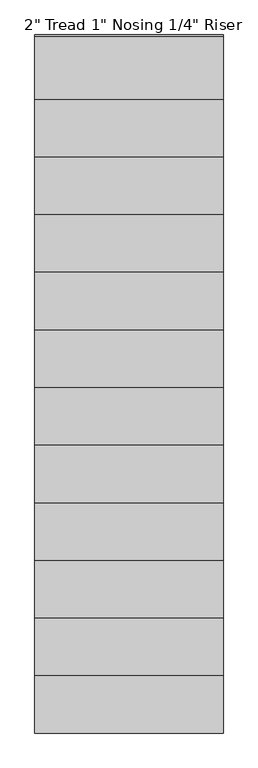
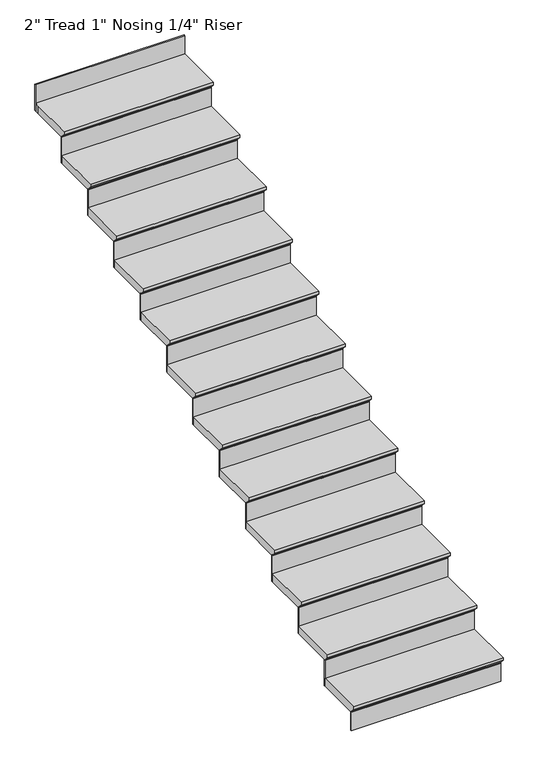
"""IFC4 building model written with IfcOpenShell, lengths in millimetres: stair flight geometry."""

from ifc_helpers import new_model, si_unit, origin, place, context, project, spatial, faceted_brep, source, transform, mapped, element, save


def stair_flight_fc83273d(model_context):
    return source(origin(), model_context, "Body", "Brep", [
        faceted_brep([(-2703.0415084, 19841.9216096, 49768.9005799), (-2703.0415084, 19841.9216096, 49787.9505799), (-3617.4415084, 19841.9216096, 49787.9505799), (-3617.4415084, 19841.9216096, 49768.9005799), (-2703.0415084, 19867.3216096, 49743.5005799), (-3617.4415084, 19867.3216096, 49743.5005799), (-2703.0415084, 20146.7216096, 49787.9505799), (-3617.4415084, 20146.7216096, 49787.9505799), (-3617.4415084, 19867.3216096, 49737.1505799), (-3617.4415084, 20146.7216096, 49737.1505799), (-2703.0415084, 20146.7216096, 49737.1505799), (-2703.0415084, 19867.3216096, 49737.1505799)], [[[0, 1, 2, 3]], [[4, 0, 3, 5]], [[2, 1, 6, 7]], [[8, 9, 10, 11]], [[2, 7, 9, 8, 5, 3]], [[8, 11, 4, 5]], [[6, 1, 0, 4, 11, 10]], [[7, 6, 10, 9]]]),
        faceted_brep([(-2703.0415084, 19867.3216096, 49737.1505799), (-2703.0415084, 19867.3216096, 49618.6172466), (-2703.0415084, 19873.6716096, 49618.6172466), (-2703.0415084, 19873.6716096, 49737.1505799), (-3617.4415084, 19867.3216096, 49737.1505799), (-3617.4415084, 19873.6716096, 49737.1505799), (-3617.4415084, 19873.6716096, 49618.6172466), (-3617.4415084, 19867.3216096, 49618.6172466)], [[[0, 1, 2, 3]], [[4, 5, 6, 7]], [[1, 0, 4, 7]], [[2, 1, 7, 6]], [[3, 2, 6, 5]], [[0, 3, 5, 4]]]),
        faceted_brep([(-2703.0415084, 20146.7216096, 49906.4839133), (-2703.0415084, 20146.7216096, 49737.1505799), (-2703.0415084, 20153.0716096, 49737.1505799), (-2703.0415084, 20153.0716096, 49906.4839133), (-3617.4415084, 20146.7216096, 49906.4839133), (-3617.4415084, 20153.0716096, 49906.4839133), (-3617.4415084, 20153.0716096, 49737.1505799), (-3617.4415084, 20146.7216096, 49737.1505799)], [[[0, 1, 2, 3]], [[4, 5, 6, 7]], [[1, 0, 4, 7]], [[2, 1, 7, 6]], [[3, 2, 6, 5]], [[0, 3, 5, 4]]]),
        faceted_brep([(-3617.4415084, 20121.3216096, 49957.2839133), (-2703.0415084, 20121.3216096, 49957.2839133), (-2703.0415084, 20426.1216096, 49957.2839133), (-3617.4415084, 20426.1216096, 49957.2839133), (-3617.4415084, 20146.7216096, 49906.4839133), (-3617.4415084, 20426.1216096, 49906.4839133), (-2703.0415084, 20426.1216096, 49906.4839133), (-2703.0415084, 20146.7216096, 49906.4839133), (-3617.4415084, 20146.7216096, 49912.8339133), (-3617.4415084, 20121.3216096, 49938.2339133), (-2703.0415084, 20146.7216096, 49912.8339133), (-2703.0415084, 20121.3216096, 49938.2339133)], [[[0, 1, 2, 3]], [[4, 5, 6, 7]], [[0, 3, 5, 4, 8, 9]], [[4, 7, 10, 8]], [[2, 1, 11, 10, 7, 6]], [[3, 2, 6, 5]], [[11, 1, 0, 9]], [[10, 11, 9, 8]]]),
        faceted_brep([(-2703.0415084, 20426.1216096, 50075.8172466), (-2703.0415084, 20426.1216096, 49906.4839133), (-2703.0415084, 20432.4716096, 49906.4839133), (-2703.0415084, 20432.4716096, 50075.8172466), (-3617.4415084, 20426.1216096, 50075.8172466), (-3617.4415084, 20432.4716096, 50075.8172466), (-3617.4415084, 20432.4716096, 49906.4839133), (-3617.4415084, 20426.1216096, 49906.4839133)], [[[0, 1, 2, 3]], [[4, 5, 6, 7]], [[1, 0, 4, 7]], [[2, 1, 7, 6]], [[3, 2, 6, 5]], [[0, 3, 5, 4]]]),
        faceted_brep([(-3617.4415084, 20400.7216096, 50126.6172466), (-2703.0415084, 20400.7216096, 50126.6172466), (-2703.0415084, 20705.5216096, 50126.6172466), (-3617.4415084, 20705.5216096, 50126.6172466), (-3617.4415084, 20426.1216096, 50075.8172466), (-3617.4415084, 20705.5216096, 50075.8172466), (-2703.0415084, 20705.5216096, 50075.8172466), (-2703.0415084, 20426.1216096, 50075.8172466), (-3617.4415084, 20426.1216096, 50082.1672466), (-3617.4415084, 20400.7216096, 50107.5672466), (-2703.0415084, 20426.1216096, 50082.1672466), (-2703.0415084, 20400.7216096, 50107.5672466)], [[[0, 1, 2, 3]], [[4, 5, 6, 7]], [[0, 3, 5, 4, 8, 9]], [[4, 7, 10, 8]], [[2, 1, 11, 10, 7, 6]], [[3, 2, 6, 5]], [[11, 1, 0, 9]], [[10, 11, 9, 8]]]),
        faceted_brep([(-2703.0415084, 20705.5216096, 50245.1505799), (-2703.0415084, 20705.5216096, 50075.8172466), (-2703.0415084, 20711.8716096, 50075.8172466), (-2703.0415084, 20711.8716096, 50245.1505799), (-3617.4415084, 20705.5216096, 50245.1505799), (-3617.4415084, 20711.8716096, 50245.1505799), (-3617.4415084, 20711.8716096, 50075.8172466), (-3617.4415084, 20705.5216096, 50075.8172466)], [[[0, 1, 2, 3]], [[4, 5, 6, 7]], [[1, 0, 4, 7]], [[2, 1, 7, 6]], [[3, 2, 6, 5]], [[0, 3, 5, 4]]]),
        faceted_brep([(-3617.4415084, 20680.1216096, 50295.9505799), (-2703.0415084, 20680.1216096, 50295.9505799), (-2703.0415084, 20984.9216096, 50295.9505799), (-3617.4415084, 20984.9216096, 50295.9505799), (-3617.4415084, 20705.5216096, 50245.1505799), (-3617.4415084, 20984.9216096, 50245.1505799), (-2703.0415084, 20984.9216096, 50245.1505799), (-2703.0415084, 20705.5216096, 50245.1505799), (-3617.4415084, 20705.5216096, 50251.5005799), (-3617.4415084, 20680.1216096, 50276.9005799), (-2703.0415084, 20705.5216096, 50251.5005799), (-2703.0415084, 20680.1216096, 50276.9005799)], [[[0, 1, 2, 3]], [[4, 5, 6, 7]], [[0, 3, 5, 4, 8, 9]], [[4, 7, 10, 8]], [[2, 1, 11, 10, 7, 6]], [[3, 2, 6, 5]], [[11, 1, 0, 9]], [[10, 11, 9, 8]]]),
        faceted_brep([(-2703.0415084, 20984.9216096, 50414.4839133), (-2703.0415084, 20984.9216096, 50245.1505799), (-2703.0415084, 20991.2716096, 50245.1505799), (-2703.0415084, 20991.2716096, 50414.4839133), (-3617.4415084, 20984.9216096, 50414.4839133), (-3617.4415084, 20991.2716096, 50414.4839133), (-3617.4415084, 20991.2716096, 50245.1505799), (-3617.4415084, 20984.9216096, 50245.1505799)], [[[0, 1, 2, 3]], [[4, 5, 6, 7]], [[1, 0, 4, 7]], [[2, 1, 7, 6]], [[3, 2, 6, 5]], [[0, 3, 5, 4]]]),
        faceted_brep([(-3617.4415084, 20959.5216096, 50465.2839133), (-2703.0415084, 20959.5216096, 50465.2839133), (-2703.0415084, 21264.3216096, 50465.2839133), (-3617.4415084, 21264.3216096, 50465.2839133), (-3617.4415084, 20984.9216096, 50414.4839133), (-3617.4415084, 21264.3216096, 50414.4839133), (-2703.0415084, 21264.3216096, 50414.4839133), (-2703.0415084, 20984.9216096, 50414.4839133), (-3617.4415084, 20984.9216096, 50420.8339133), (-3617.4415084, 20959.5216096, 50446.2339133), (-2703.0415084, 20984.9216096, 50420.8339133), (-2703.0415084, 20959.5216096, 50446.2339133)], [[[0, 1, 2, 3]], [[4, 5, 6, 7]], [[0, 3, 5, 4, 8, 9]], [[4, 7, 10, 8]], [[2, 1, 11, 10, 7, 6]], [[3, 2, 6, 5]], [[11, 1, 0, 9]], [[10, 11, 9, 8]]]),
        faceted_brep([(-2703.0415084, 21264.3216096, 50583.8172466), (-2703.0415084, 21264.3216096, 50414.4839133), (-2703.0415084, 21270.6716096, 50414.4839133), (-2703.0415084, 21270.6716096, 50583.8172466), (-3617.4415084, 21264.3216096, 50583.8172466), (-3617.4415084, 21270.6716096, 50583.8172466), (-3617.4415084, 21270.6716096, 50414.4839133), (-3617.4415084, 21264.3216096, 50414.4839133)], [[[0, 1, 2, 3]], [[4, 5, 6, 7]], [[1, 0, 4, 7]], [[2, 1, 7, 6]], [[3, 2, 6, 5]], [[0, 3, 5, 4]]]),
        faceted_brep([(-3617.4415084, 21238.9216096, 50634.6172466), (-2703.0415084, 21238.9216096, 50634.6172466), (-2703.0415084, 21543.7216096, 50634.6172466), (-3617.4415084, 21543.7216096, 50634.6172466), (-3617.4415084, 21264.3216096, 50583.8172466), (-3617.4415084, 21543.7216096, 50583.8172466), (-2703.0415084, 21543.7216096, 50583.8172466), (-2703.0415084, 21264.3216096, 50583.8172466), (-3617.4415084, 21264.3216096, 50590.1672466), (-3617.4415084, 21238.9216096, 50615.5672466), (-2703.0415084, 21264.3216096, 50590.1672466), (-2703.0415084, 21238.9216096, 50615.5672466)], [[[0, 1, 2, 3]], [[4, 5, 6, 7]], [[0, 3, 5, 4, 8, 9]], [[4, 7, 10, 8]], [[2, 1, 11, 10, 7, 6]], [[3, 2, 6, 5]], [[11, 1, 0, 9]], [[10, 11, 9, 8]]]),
        faceted_brep([(-2703.0415084, 21543.7216096, 50753.1505799), (-2703.0415084, 21543.7216096, 50583.8172466), (-2703.0415084, 21550.0716096, 50583.8172466), (-2703.0415084, 21550.0716096, 50753.1505799), (-3617.4415084, 21543.7216096, 50753.1505799), (-3617.4415084, 21550.0716096, 50753.1505799), (-3617.4415084, 21550.0716096, 50583.8172466), (-3617.4415084, 21543.7216096, 50583.8172466)], [[[0, 1, 2, 3]], [[4, 5, 6, 7]], [[1, 0, 4, 7]], [[2, 1, 7, 6]], [[3, 2, 6, 5]], [[0, 3, 5, 4]]]),
        faceted_brep([(-3617.4415084, 21518.3216096, 50803.9505799), (-2703.0415084, 21518.3216096, 50803.9505799), (-2703.0415084, 21823.1216096, 50803.9505799), (-3617.4415084, 21823.1216096, 50803.9505799), (-3617.4415084, 21543.7216096, 50753.1505799), (-3617.4415084, 21823.1216096, 50753.1505799), (-2703.0415084, 21823.1216096, 50753.1505799), (-2703.0415084, 21543.7216096, 50753.1505799), (-3617.4415084, 21543.7216096, 50759.5005799), (-3617.4415084, 21518.3216096, 50784.9005799), (-2703.0415084, 21543.7216096, 50759.5005799), (-2703.0415084, 21518.3216096, 50784.9005799)], [[[0, 1, 2, 3]], [[4, 5, 6, 7]], [[0, 3, 5, 4, 8, 9]], [[4, 7, 10, 8]], [[2, 1, 11, 10, 7, 6]], [[3, 2, 6, 5]], [[11, 1, 0, 9]], [[10, 11, 9, 8]]]),
        faceted_brep([(-2703.0415084, 21823.1216096, 50922.4839133), (-2703.0415084, 21823.1216096, 50753.1505799), (-2703.0415084, 21829.4716096, 50753.1505799), (-2703.0415084, 21829.4716096, 50922.4839133), (-3617.4415084, 21823.1216096, 50922.4839133), (-3617.4415084, 21829.4716096, 50922.4839133), (-3617.4415084, 21829.4716096, 50753.1505799), (-3617.4415084, 21823.1216096, 50753.1505799)], [[[0, 1, 2, 3]], [[4, 5, 6, 7]], [[1, 0, 4, 7]], [[2, 1, 7, 6]], [[3, 2, 6, 5]], [[0, 3, 5, 4]]]),
        faceted_brep([(-3617.4415084, 21797.7216096, 50973.2839133), (-2703.0415084, 21797.7216096, 50973.2839133), (-2703.0415084, 22102.5216096, 50973.2839133), (-3617.4415084, 22102.5216096, 50973.2839133), (-3617.4415084, 21823.1216096, 50922.4839133), (-3617.4415084, 22102.5216096, 50922.4839133), (-2703.0415084, 22102.5216096, 50922.4839133), (-2703.0415084, 21823.1216096, 50922.4839133), (-3617.4415084, 21823.1216096, 50928.8339133), (-3617.4415084, 21797.7216096, 50954.2339133), (-2703.0415084, 21823.1216096, 50928.8339133), (-2703.0415084, 21797.7216096, 50954.2339133)], [[[0, 1, 2, 3]], [[4, 5, 6, 7]], [[0, 3, 5, 4, 8, 9]], [[4, 7, 10, 8]], [[2, 1, 11, 10, 7, 6]], [[3, 2, 6, 5]], [[11, 1, 0, 9]], [[10, 11, 9, 8]]]),
        faceted_brep([(-2703.0415084, 22102.5216096, 51091.8172466), (-2703.0415084, 22102.5216096, 50922.4839133), (-2703.0415084, 22108.8716096, 50922.4839133), (-2703.0415084, 22108.8716096, 51091.8172466), (-3617.4415084, 22102.5216096, 51091.8172466), (-3617.4415084, 22108.8716096, 51091.8172466), (-3617.4415084, 22108.8716096, 50922.4839133), (-3617.4415084, 22102.5216096, 50922.4839133)], [[[0, 1, 2, 3]], [[4, 5, 6, 7]], [[1, 0, 4, 7]], [[2, 1, 7, 6]], [[3, 2, 6, 5]], [[0, 3, 5, 4]]]),
        faceted_brep([(-3617.4415084, 22077.1216096, 51142.6172466), (-2703.0415084, 22077.1216096, 51142.6172466), (-2703.0415084, 22381.9216096, 51142.6172466), (-3617.4415084, 22381.9216096, 51142.6172466), (-3617.4415084, 22102.5216096, 51091.8172466), (-3617.4415084, 22381.9216096, 51091.8172466), (-2703.0415084, 22381.9216096, 51091.8172466), (-2703.0415084, 22102.5216096, 51091.8172466), (-3617.4415084, 22102.5216096, 51098.1672466), (-3617.4415084, 22077.1216096, 51123.5672466), (-2703.0415084, 22102.5216096, 51098.1672466), (-2703.0415084, 22077.1216096, 51123.5672466)], [[[0, 1, 2, 3]], [[4, 5, 6, 7]], [[0, 3, 5, 4, 8, 9]], [[4, 7, 10, 8]], [[2, 1, 11, 10, 7, 6]], [[3, 2, 6, 5]], [[11, 1, 0, 9]], [[10, 11, 9, 8]]]),
        faceted_brep([(-2703.0415084, 22381.9216096, 51261.1505799), (-2703.0415084, 22381.9216096, 51091.8172466), (-2703.0415084, 22388.2716096, 51091.8172466), (-2703.0415084, 22388.2716096, 51261.1505799), (-3617.4415084, 22381.9216096, 51261.1505799), (-3617.4415084, 22388.2716096, 51261.1505799), (-3617.4415084, 22388.2716096, 51091.8172466), (-3617.4415084, 22381.9216096, 51091.8172466)], [[[0, 1, 2, 3]], [[4, 5, 6, 7]], [[1, 0, 4, 7]], [[2, 1, 7, 6]], [[3, 2, 6, 5]], [[0, 3, 5, 4]]]),
        faceted_brep([(-3617.4415084, 22356.5216096, 51311.9505799), (-2703.0415084, 22356.5216096, 51311.9505799), (-2703.0415084, 22661.3216096, 51311.9505799), (-3617.4415084, 22661.3216096, 51311.9505799), (-3617.4415084, 22381.9216096, 51261.1505799), (-3617.4415084, 22661.3216096, 51261.1505799), (-2703.0415084, 22661.3216096, 51261.1505799), (-2703.0415084, 22381.9216096, 51261.1505799), (-3617.4415084, 22381.9216096, 51267.5005799), (-3617.4415084, 22356.5216096, 51292.9005799), (-2703.0415084, 22381.9216096, 51267.5005799), (-2703.0415084, 22356.5216096, 51292.9005799)], [[[0, 1, 2, 3]], [[4, 5, 6, 7]], [[0, 3, 5, 4, 8, 9]], [[4, 7, 10, 8]], [[2, 1, 11, 10, 7, 6]], [[3, 2, 6, 5]], [[11, 1, 0, 9]], [[10, 11, 9, 8]]]),
        faceted_brep([(-2703.0415084, 22661.3216096, 51430.4839133), (-2703.0415084, 22661.3216096, 51261.1505799), (-2703.0415084, 22667.6716096, 51261.1505799), (-2703.0415084, 22667.6716096, 51430.4839133), (-3617.4415084, 22661.3216096, 51430.4839133), (-3617.4415084, 22667.6716096, 51430.4839133), (-3617.4415084, 22667.6716096, 51261.1505799), (-3617.4415084, 22661.3216096, 51261.1505799)], [[[0, 1, 2, 3]], [[4, 5, 6, 7]], [[1, 0, 4, 7]], [[2, 1, 7, 6]], [[3, 2, 6, 5]], [[0, 3, 5, 4]]]),
        faceted_brep([(-3617.4415084, 22635.9216096, 51481.2839133), (-2703.0415084, 22635.9216096, 51481.2839133), (-2703.0415084, 22940.7216096, 51481.2839133), (-3617.4415084, 22940.7216096, 51481.2839133), (-3617.4415084, 22661.3216096, 51430.4839133), (-3617.4415084, 22940.7216096, 51430.4839133), (-2703.0415084, 22940.7216096, 51430.4839133), (-2703.0415084, 22661.3216096, 51430.4839133), (-3617.4415084, 22661.3216096, 51436.8339133), (-3617.4415084, 22635.9216096, 51462.2339133), (-2703.0415084, 22661.3216096, 51436.8339133), (-2703.0415084, 22635.9216096, 51462.2339133)], [[[0, 1, 2, 3]], [[4, 5, 6, 7]], [[0, 3, 5, 4, 8, 9]], [[4, 7, 10, 8]], [[2, 1, 11, 10, 7, 6]], [[3, 2, 6, 5]], [[11, 1, 0, 9]], [[10, 11, 9, 8]]]),
        faceted_brep([(-2703.0415084, 23220.1216096, 51769.1505799), (-2703.0415084, 23220.1216096, 51599.8172466), (-2703.0415084, 23226.4716096, 51599.8172466), (-2703.0415084, 23226.4716096, 51769.1505799), (-3617.4415084, 23220.1216096, 51769.1505799), (-3617.4415084, 23226.4716096, 51769.1505799), (-3617.4415084, 23226.4716096, 51599.8172466), (-3617.4415084, 23220.1216096, 51599.8172466)], [[[0, 1, 2, 3]], [[4, 5, 6, 7]], [[1, 0, 4, 7]], [[2, 1, 7, 6]], [[3, 2, 6, 5]], [[0, 3, 5, 4]]]),
        faceted_brep([(-2703.0415084, 22940.7216096, 51599.8172466), (-2703.0415084, 22940.7216096, 51430.4839133), (-2703.0415084, 22947.0716096, 51430.4839133), (-2703.0415084, 22947.0716096, 51599.8172466), (-3617.4415084, 22940.7216096, 51599.8172466), (-3617.4415084, 22947.0716096, 51599.8172466), (-3617.4415084, 22947.0716096, 51430.4839133), (-3617.4415084, 22940.7216096, 51430.4839133)], [[[0, 1, 2, 3]], [[4, 5, 6, 7]], [[1, 0, 4, 7]], [[2, 1, 7, 6]], [[3, 2, 6, 5]], [[0, 3, 5, 4]]]),
        faceted_brep([(-3617.4415084, 23220.1216096, 51650.6172466), (-3617.4415084, 23194.7216096, 51650.6172466), (-3617.4415084, 22915.3216096, 51650.6172466), (-2703.0415084, 22915.3216096, 51650.6172466), (-2703.0415084, 23220.1216096, 51650.6172466), (-3617.4415084, 23194.7216096, 51599.8172466), (-3617.4415084, 23220.1216096, 51599.8172466), (-2703.0415084, 23220.1216096, 51599.8172466), (-2703.0415084, 22940.7216096, 51599.8172466), (-3617.4415084, 22940.7216096, 51599.8172466), (-3617.4415084, 22940.7216096, 51606.1672466), (-3617.4415084, 22915.3216096, 51631.5672466), (-2703.0415084, 22940.7216096, 51606.1672466), (-2703.0415084, 22915.3216096, 51631.5672466)], [[[0, 1, 2, 3, 4]], [[5, 6, 7, 8, 9]], [[1, 0, 6, 5]], [[2, 1, 5, 9, 10, 11]], [[9, 8, 12, 10]], [[4, 3, 13, 12, 8, 7]], [[0, 4, 7, 6]], [[13, 3, 2, 11]], [[12, 13, 11, 10]]]),
    ])


if __name__ == "__main__":
    model = new_model("IFC4")
    model_context = context("Model", 3, world=origin())
    ifc_project = project(units=[si_unit("LENGTHUNIT", "METRE", prefix="MILLI")], contexts=[model_context])
    site = spatial("IfcSite", under=ifc_project)
    building = spatial("IfcBuilding", under=site)
    placement = place(None, origin())
    stair_flight_shape = stair_flight_fc83273d(model_context)
    element("IfcStairFlight", 1, ObjectType="2\" Tread 1\" Nosing 1/4\" Riser", at=placement, inside=building, context=model_context, shape_type="MappedRepresentation", body=[
        mapped(stair_flight_shape, transform((0.0, 0.0, 0.0), x_axis=(1.0, 0.0, 0.0), y_axis=(0.0, 1.0, 0.0), z_axis=(0.0, 0.0, 1.0))),
    ])
    save(model, "model.ifc")
